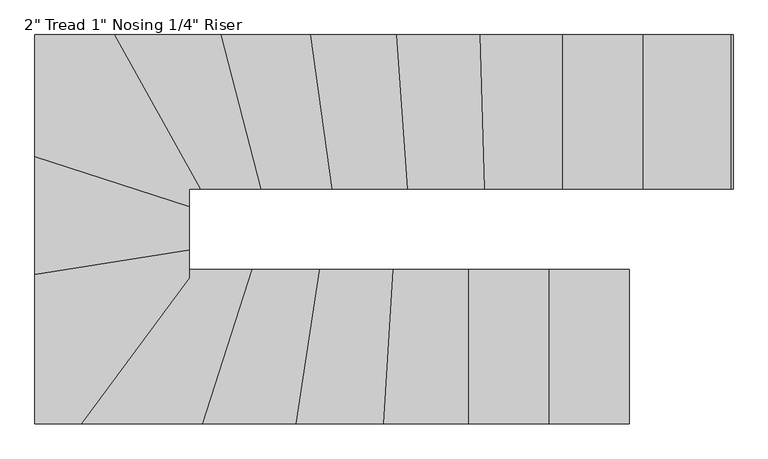
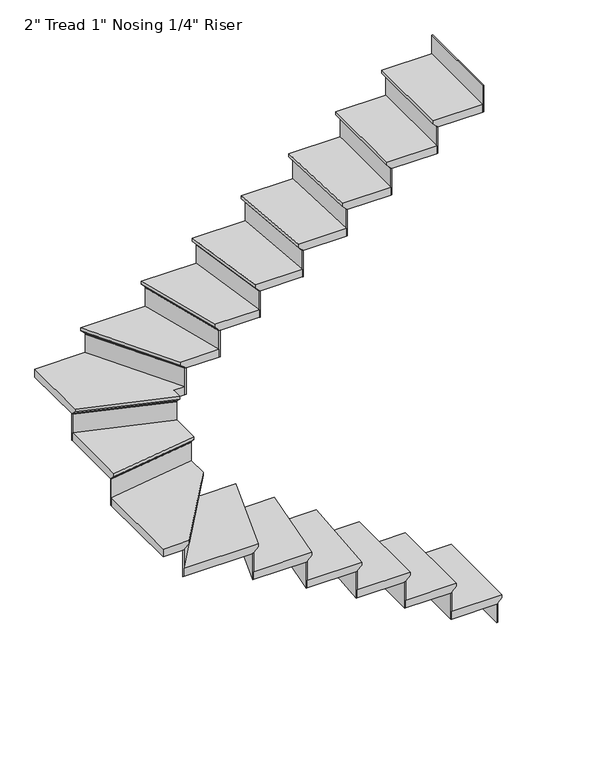
"""IFC4 building model written with IfcOpenShell, lengths in millimetres: stair flight geometry."""

from ifc_helpers import new_model, si_unit, origin, place, context, project, spatial, faceted_brep, source, transform, mapped, element, save


def stair_flight_033e9654(model_context):
    return source(origin(), model_context, "Body", "Brep", [
        faceted_brep([(-264.8831579, 264.4433073, 6551.0833333), (-264.8831579, 264.4433073, 6570.1333333), (-264.8831579, -271.8029286, 6570.1333333), (-264.8831579, -271.8029286, 6551.0833333), (-290.2831579, 264.4433073, 6525.6833333), (-290.2831579, -271.8029286, 6525.6833333), (-569.6831579, 264.4433073, 6570.1333333), (-569.6831579, -271.8029286, 6570.1333333), (-290.2831579, -271.8029286, 6519.3333333), (-569.6831579, -271.8029286, 6519.3333333), (-569.6831579, 264.4433073, 6519.3333333), (-290.2831579, 264.4433073, 6519.3333333)], [[[0, 1, 2, 3]], [[4, 0, 3, 5]], [[2, 1, 6, 7]], [[8, 9, 10, 11]], [[2, 7, 9, 8, 5, 3]], [[8, 11, 4, 5]], [[6, 1, 0, 4, 11, 10]], [[7, 6, 10, 9]]]),
        faceted_brep([(-290.2831579, 264.4433073, 6519.3333333), (-290.2831579, 264.4433073, 6400.8), (-296.6331579, 264.4433073, 6400.8), (-296.6331579, 264.4433073, 6519.3333333), (-290.2831579, -271.8029286, 6519.3333333), (-296.6331579, -271.8029286, 6519.3333333), (-296.6331579, -271.8029286, 6400.8), (-290.2831579, -271.8029286, 6400.8)], [[[0, 1, 2, 3]], [[4, 5, 6, 7]], [[1, 0, 4, 7]], [[2, 1, 7, 6]], [[3, 2, 6, 5]], [[0, 3, 5, 4]]]),
        faceted_brep([(-569.6831579, 264.4433073, 6688.6666667), (-569.6831579, 264.4433073, 6519.3333333), (-576.0331579, 264.4433073, 6519.3333333), (-576.0331579, 264.4433073, 6688.6666667), (-569.6831579, -271.8029286, 6688.6666667), (-576.0331579, -271.8029286, 6688.6666667), (-576.0331579, -271.8029286, 6519.3333333), (-569.6831579, -271.8029286, 6519.3333333)], [[[0, 1, 2, 3]], [[4, 5, 6, 7]], [[1, 0, 4, 7]], [[2, 1, 7, 6]], [[3, 2, 6, 5]], [[0, 3, 5, 4]]]),
        faceted_brep([(-544.2831579, -271.8029286, 6739.4666667), (-544.2831579, 264.4433073, 6739.4666667), (-849.0831579, 264.4433073, 6739.4666667), (-849.0831579, -271.8029286, 6739.4666667), (-569.6831579, -271.8029286, 6688.6666667), (-849.0831579, -271.8029286, 6688.6666667), (-849.0831579, 264.4433073, 6688.6666667), (-569.6831579, 264.4433073, 6688.6666667), (-569.6831579, -271.8029286, 6695.0166667), (-544.2831579, -271.8029286, 6720.4166667), (-569.6831579, 264.4433073, 6695.0166667), (-544.2831579, 264.4433073, 6720.4166667)], [[[0, 1, 2, 3]], [[4, 5, 6, 7]], [[0, 3, 5, 4, 8, 9]], [[4, 7, 10, 8]], [[2, 1, 11, 10, 7, 6]], [[3, 2, 6, 5]], [[11, 1, 0, 9]], [[10, 11, 9, 8]]]),
        faceted_brep([(-849.0831579, 264.4433073, 6858.0), (-849.0831579, 264.4433073, 6688.6666667), (-855.4331579, 264.4433073, 6688.6666667), (-855.4331579, 264.4433073, 6858.0), (-849.0831579, -271.8029286, 6858.0), (-855.4331579, -271.8029286, 6858.0), (-855.4331579, -271.8029286, 6688.6666667), (-849.0831579, -271.8029286, 6688.6666667)], [[[0, 1, 2, 3]], [[4, 5, 6, 7]], [[1, 0, 4, 7]], [[2, 1, 7, 6]], [[3, 2, 6, 5]], [[0, 3, 5, 4]]]),
        faceted_brep([(-823.6831579, -271.8029286, 6908.8), (-823.6831579, 264.4433073, 6908.8), (-1112.6009003, 264.4433073, 6908.8), (-1144.4549627, -271.8029286, 6908.8), (-849.0831579, -271.8029286, 6858.0), (-1144.4549627, -271.8029286, 6858.0), (-1112.6009003, 264.4433073, 6858.0), (-849.0831579, 264.4433073, 6858.0), (-849.0831579, -271.8029286, 6864.35), (-823.6831579, -271.8029286, 6889.75), (-849.0831579, 264.4433073, 6864.35), (-823.6831579, 264.4433073, 6889.75)], [[[0, 1, 2, 3]], [[4, 5, 6, 7]], [[0, 3, 5, 4, 8, 9]], [[4, 7, 10, 8]], [[2, 1, 11, 10, 7, 6]], [[3, 2, 6, 5]], [[11, 1, 0, 9]], [[10, 11, 9, 8]]]),
        faceted_brep([(-1112.6009003, 264.4433073, 7027.3333333), (-1112.6009003, 264.4433073, 6858.0), (-1118.9620938, 264.4433073, 6858.0), (-1118.9620938, 264.4433073, 7027.3333333), (-1144.4549627, -271.8029286, 7027.3333333), (-1150.8161561, -271.8029286, 7027.3333333), (-1150.8161561, -271.8029286, 6858.0), (-1144.4549627, -271.8029286, 6858.0)], [[[0, 1, 2, 3]], [[4, 5, 6, 7]], [[1, 0, 4, 7]], [[2, 1, 7, 6]], [[3, 2, 6, 5]], [[0, 3, 5, 4]]]),
        faceted_brep([(-1119.0101891, -271.8029286, 7078.1333333), (-1087.1561267, 264.4433073, 7078.1333333), (-1367.1376579, 264.4433073, 7078.1333333), (-1449.2203373, -271.8029286, 7078.1333333), (-1144.4549627, -271.8029286, 7027.3333333), (-1449.2203373, -271.8029286, 7027.3333333), (-1367.1376579, 264.4433073, 7027.3333333), (-1112.6009003, 264.4433073, 7027.3333333), (-1144.4549627, -271.8029286, 7033.6833333), (-1119.0101891, -271.8029286, 7059.0833333), (-1112.6009003, 264.4433073, 7033.6833333), (-1087.1561267, 264.4433073, 7059.0833333)], [[[0, 1, 2, 3]], [[4, 5, 6, 7]], [[0, 3, 5, 4, 8, 9]], [[4, 7, 10, 8]], [[2, 1, 11, 10, 7, 6]], [[3, 2, 6, 5]], [[11, 1, 0, 9]], [[10, 11, 9, 8]]]),
        faceted_brep([(-1367.1376579, 264.4433073, 7196.6666667), (-1367.1376579, 264.4433073, 7027.3333333), (-1373.5616178, 264.4433073, 7027.3333333), (-1373.5616178, 264.4433073, 7196.6666667), (-1449.2203373, -271.8029286, 7196.6666667), (-1455.6442972, -271.8029286, 7196.6666667), (-1455.6442972, -271.8029286, 7027.3333333), (-1449.2203373, -271.8029286, 7027.3333333)], [[[0, 1, 2, 3]], [[4, 5, 6, 7]], [[1, 0, 4, 7]], [[2, 1, 7, 6]], [[3, 2, 6, 5]], [[0, 3, 5, 4]]]),
        faceted_brep([(-1423.5244976, -271.8029286, 7247.4666667), (-1341.4418182, 264.4433073, 7247.4666667), (-1602.0584075, 264.4433073, 7247.4666667), (-1775.0869242, -271.8029286, 7247.4666667), (-1449.2203373, -271.8029286, 7196.6666667), (-1775.0869242, -271.8029286, 7196.6666667), (-1602.0584075, 264.4433073, 7196.6666667), (-1367.1376579, 264.4433073, 7196.6666667), (-1449.2203373, -271.8029286, 7203.0166667), (-1423.5244976, -271.8029286, 7228.4166667), (-1367.1376579, 264.4433073, 7203.0166667), (-1341.4418182, 264.4433073, 7228.4166667)], [[[0, 1, 2, 3]], [[4, 5, 6, 7]], [[0, 3, 5, 4, 8, 9]], [[4, 7, 10, 8]], [[2, 1, 11, 10, 7, 6]], [[3, 2, 6, 5]], [[11, 1, 0, 9]], [[10, 11, 9, 8]]]),
        faceted_brep([(-1602.0584075, 264.4433073, 7366.0), (-1602.0584075, 264.4433073, 7196.6666667), (-1608.7307845, 264.4433073, 7196.6666667), (-1608.7307845, 264.4433073, 7366.0), (-1775.0869242, -271.8029286, 7366.0), (-1781.7593012, -271.8029286, 7366.0), (-1781.7593012, -271.8029286, 7196.6666667), (-1775.0869242, -271.8029286, 7196.6666667)], [[[0, 1, 2, 3]], [[4, 5, 6, 7]], [[1, 0, 4, 7]], [[2, 1, 7, 6]], [[3, 2, 6, 5]], [[0, 3, 5, 4]]]),
        faceted_brep([(-1748.3974163, -271.8029286, 7416.8), (-1575.3688995, 264.4433073, 7416.8), (-1792.6148498, 264.4433073, 7416.8), (-1792.6148498, 277.721026, 7416.8), (-2200.2950016, -271.8029286, 7416.8), (-1775.0869242, -271.8029286, 7366.0), (-2200.2950016, -271.8029286, 7366.0), (-1792.6148498, 277.721026, 7366.0), (-1792.6148498, 264.4433073, 7366.0), (-1602.0584075, 264.4433073, 7366.0), (-1775.0869242, -271.8029286, 7372.35), (-1748.3974163, -271.8029286, 7397.75), (-1602.0584075, 264.4433073, 7372.35), (-1575.3688995, 264.4433073, 7397.75)], [[[0, 1, 2, 3, 4]], [[5, 6, 7, 8, 9]], [[0, 4, 6, 5, 10, 11]], [[5, 9, 12, 10]], [[2, 1, 13, 12, 9, 8]], [[4, 3, 7, 6]], [[13, 1, 0, 11]], [[12, 13, 11, 10]], [[3, 2, 8, 7]]]),
        faceted_brep([(-1792.6148498, 277.721026, 7535.3333333), (-1792.6148498, 277.721026, 7366.0), (-1792.6148498, 288.3786511, 7366.0), (-1792.6148498, 288.3786511, 7535.3333333), (-2200.2950016, -271.8029286, 7535.3333333), (-2208.2016673, -271.8029286, 7535.3333333), (-2208.2016673, -271.8029286, 7366.0), (-2200.2950016, -271.8029286, 7366.0)], [[[0, 1, 2, 3]], [[4, 5, 6, 7]], [[1, 0, 4, 7]], [[2, 1, 7, 6]], [[3, 2, 6, 5]], [[0, 3, 5, 4]]]),
        faceted_brep([(-2328.8610857, 272.9225747, 7586.1333333), (-2328.8610857, -271.8029286, 7586.1333333), (-2168.6683387, -271.8029286, 7586.1333333), (-1792.6148498, 235.0905257, 7586.1333333), (-1792.6148498, 358.7948785, 7586.1333333), (-2328.8610857, -271.8029286, 7535.3333333), (-2328.8610857, 272.9225747, 7535.3333333), (-1792.6148498, 358.7948785, 7535.3333333), (-1792.6148498, 277.721026, 7535.3333333), (-2200.2950016, -271.8029286, 7535.3333333), (-2200.2950016, -271.8029286, 7541.6833333), (-2168.6683387, -271.8029286, 7567.0833333), (-1792.6148498, 277.721026, 7541.6833333), (-1792.6148498, 235.0905257, 7567.0833333)], [[[0, 1, 2, 3, 4]], [[5, 6, 7, 8, 9]], [[1, 0, 6, 5]], [[2, 1, 5, 9, 10, 11]], [[9, 8, 12, 10]], [[4, 3, 13, 12, 8, 7]], [[0, 4, 7, 6]], [[13, 3, 2, 11]], [[12, 13, 11, 10]]]),
        faceted_brep([(-1792.6148498, 358.7948785, 7704.6666667), (-1792.6148498, 358.7948785, 7535.3333333), (-1792.6148498, 365.2257813, 7535.3333333), (-1792.6148498, 365.2257813, 7704.6666667), (-2328.8610857, 272.9225747, 7704.6666667), (-2328.8610857, 279.3534775, 7704.6666667), (-2328.8610857, 279.3534775, 7535.3333333), (-2328.8610857, 272.9225747, 7535.3333333)], [[[0, 1, 2, 3]], [[4, 5, 6, 7]], [[1, 0, 4, 7]], [[2, 1, 7, 6]], [[3, 2, 6, 5]], [[0, 3, 5, 4]]]),
        faceted_brep([(-2328.8610857, 247.1989634, 7755.4666667), (-1792.6148498, 333.0712672, 7755.4666667), (-1792.6148498, 510.0383883, 7755.4666667), (-2328.8610857, 683.2061106, 7755.4666667), (-2328.8610857, 272.9225747, 7704.6666667), (-2328.8610857, 683.2061106, 7704.6666667), (-1792.6148498, 510.0383883, 7704.6666667), (-1792.6148498, 358.7948785, 7704.6666667), (-2328.8610857, 272.9225747, 7711.0166667), (-2328.8610857, 247.1989634, 7736.4166667), (-1792.6148498, 358.7948785, 7711.0166667), (-1792.6148498, 333.0712672, 7736.4166667)], [[[0, 1, 2, 3]], [[4, 5, 6, 7]], [[0, 3, 5, 4, 8, 9]], [[4, 7, 10, 8]], [[3, 2, 6, 5]], [[11, 1, 0, 9]], [[10, 11, 9, 8]], [[2, 1, 11, 10, 7, 6]]]),
        faceted_brep([(-1792.6148498, 510.0383883, 7874.0), (-1792.6148498, 510.0383883, 7704.6666667), (-1792.6148498, 516.7112716, 7704.6666667), (-1792.6148498, 516.7112716, 7874.0), (-2328.8610857, 683.2061106, 7874.0), (-2328.8610857, 689.878994, 7874.0), (-2328.8610857, 689.878994, 7704.6666667), (-2328.8610857, 683.2061106, 7704.6666667)], [[[0, 1, 2, 3]], [[4, 5, 6, 7]], [[1, 0, 4, 7]], [[2, 1, 7, 6]], [[3, 2, 6, 5]], [[0, 3, 5, 4]]]),
        faceted_brep([(-2021.9568272, 1080.0895433, 7924.8), (-2328.8610857, 1080.0895433, 7924.8), (-2328.8610857, 656.5145772, 7924.8), (-1792.6148498, 483.3468548, 7924.8), (-1792.6148498, 543.8433073, 7924.8), (-1724.5287393, 543.8433073, 7924.8), (-2328.8610857, 1080.0895433, 7874.0), (-2021.9568272, 1080.0895433, 7874.0), (-1724.5287393, 543.8433073, 7874.0), (-1792.6148498, 543.8433073, 7874.0), (-1792.6148498, 510.0383883, 7874.0), (-2328.8610857, 683.2061106, 7874.0), (-1792.6148498, 510.0383883, 7880.35), (-2328.8610857, 683.2061106, 7880.35), (-1792.6148498, 483.3468548, 7905.75), (-2328.8610857, 656.5145772, 7905.75)], [[[0, 1, 2, 3, 4, 5]], [[6, 7, 8, 9, 10, 11]], [[1, 0, 7, 6]], [[11, 10, 12, 13]], [[4, 3, 14, 12, 10, 9]], [[0, 5, 8, 7]], [[14, 3, 2, 15]], [[12, 14, 15, 13]], [[2, 1, 6, 11, 13, 15]], [[5, 4, 9, 8]]]),
        faceted_brep([(-1724.5287393, 543.8433073, 8043.3333333), (-1724.5287393, 543.8433073, 7874.0), (-1717.2673962, 543.8433073, 7874.0), (-1717.2673962, 543.8433073, 8043.3333333), (-2021.9568272, 1080.0895433, 8043.3333333), (-2014.6954841, 1080.0895433, 8043.3333333), (-2014.6954841, 1080.0895433, 7874.0), (-2021.9568272, 1080.0895433, 7874.0)], [[[0, 1, 2, 3]], [[4, 5, 6, 7]], [[1, 0, 4, 7]], [[2, 1, 7, 6]], [[3, 2, 6, 5]], [[0, 3, 5, 4]]]),
        faceted_brep([(-2051.0021996, 1080.0895433, 8094.1333333), (-1753.5741117, 543.8433073, 8094.1333333), (-1517.487325, 543.8433073, 8094.1333333), (-1656.0375972, 1080.0895433, 8094.1333333), (-2021.9568272, 1080.0895433, 8043.3333333), (-1656.0375972, 1080.0895433, 8043.3333333), (-1517.487325, 543.8433073, 8043.3333333), (-1724.5287393, 543.8433073, 8043.3333333), (-2021.9568272, 1080.0895433, 8049.6833333), (-2051.0021996, 1080.0895433, 8075.0833333), (-1724.5287393, 543.8433073, 8049.6833333), (-1753.5741117, 543.8433073, 8075.0833333)], [[[0, 1, 2, 3]], [[4, 5, 6, 7]], [[0, 3, 5, 4, 8, 9]], [[4, 7, 10, 8]], [[2, 1, 11, 10, 7, 6]], [[3, 2, 6, 5]], [[11, 1, 0, 9]], [[10, 11, 9, 8]]]),
        faceted_brep([(-1517.487325, 543.8433073, 8212.6666667), (-1517.487325, 543.8433073, 8043.3333333), (-1510.9288005, 543.8433073, 8043.3333333), (-1510.9288005, 543.8433073, 8212.6666667), (-1656.0375972, 1080.0895433, 8212.6666667), (-1649.4790727, 1080.0895433, 8212.6666667), (-1649.4790727, 1080.0895433, 8043.3333333), (-1656.0375972, 1080.0895433, 8043.3333333)], [[[0, 1, 2, 3]], [[4, 5, 6, 7]], [[1, 0, 4, 7]], [[2, 1, 7, 6]], [[3, 2, 6, 5]], [[0, 3, 5, 4]]]),
        faceted_brep([(-1682.2716952, 1080.0895433, 8263.4666667), (-1543.721423, 543.8433073, 8263.4666667), (-1271.2041837, 543.8433073, 8263.4666667), (-1344.713853, 1080.0895433, 8263.4666667), (-1656.0375972, 1080.0895433, 8212.6666667), (-1344.713853, 1080.0895433, 8212.6666667), (-1271.2041837, 543.8433073, 8212.6666667), (-1517.487325, 543.8433073, 8212.6666667), (-1656.0375972, 1080.0895433, 8219.0166667), (-1682.2716952, 1080.0895433, 8244.4166667), (-1517.487325, 543.8433073, 8219.0166667), (-1543.721423, 543.8433073, 8244.4166667)], [[[0, 1, 2, 3]], [[4, 5, 6, 7]], [[0, 3, 5, 4, 8, 9]], [[4, 7, 10, 8]], [[2, 1, 11, 10, 7, 6]], [[3, 2, 6, 5]], [[11, 1, 0, 9]], [[10, 11, 9, 8]]]),
        faceted_brep([(-1271.2041837, 543.8433073, 8382.0), (-1271.2041837, 543.8433073, 8212.6666667), (-1264.7947985, 543.8433073, 8212.6666667), (-1264.7947985, 543.8433073, 8382.0), (-1344.713853, 1080.0895433, 8382.0), (-1338.3044678, 1080.0895433, 8382.0), (-1338.3044678, 1080.0895433, 8212.6666667), (-1344.713853, 1080.0895433, 8212.6666667)], [[[0, 1, 2, 3]], [[4, 5, 6, 7]], [[1, 0, 4, 7]], [[2, 1, 7, 6]], [[3, 2, 6, 5]], [[0, 3, 5, 4]]]),
        faceted_brep([(-1370.3513937, 1080.0895433, 8432.8), (-1296.8417245, 543.8433073, 8432.8), (-1009.7763573, 543.8433073, 8432.8), (-1047.6899509, 1080.0895433, 8432.8), (-1344.713853, 1080.0895433, 8382.0), (-1047.6899509, 1080.0895433, 8382.0), (-1009.7763573, 543.8433073, 8382.0), (-1271.2041837, 543.8433073, 8382.0), (-1344.713853, 1080.0895433, 8388.35), (-1370.3513937, 1080.0895433, 8413.75), (-1271.2041837, 543.8433073, 8388.35), (-1296.8417245, 543.8433073, 8413.75)], [[[0, 1, 2, 3]], [[4, 5, 6, 7]], [[0, 3, 5, 4, 8, 9]], [[4, 7, 10, 8]], [[2, 1, 11, 10, 7, 6]], [[3, 2, 6, 5]], [[11, 1, 0, 9]], [[10, 11, 9, 8]]]),
        faceted_brep([(-1009.7763573, 543.8433073, 8551.3333333), (-1009.7763573, 543.8433073, 8382.0), (-1003.4105061, 543.8433073, 8382.0), (-1003.4105061, 543.8433073, 8551.3333333), (-1047.6899509, 1080.0895433, 8551.3333333), (-1041.3240997, 1080.0895433, 8551.3333333), (-1041.3240997, 1080.0895433, 8382.0), (-1047.6899509, 1080.0895433, 8382.0)], [[[0, 1, 2, 3]], [[4, 5, 6, 7]], [[1, 0, 4, 7]], [[2, 1, 7, 6]], [[3, 2, 6, 5]], [[0, 3, 5, 4]]]),
        faceted_brep([(-1073.1533559, 1080.0895433, 8602.1333333), (-1035.2397623, 543.8433073, 8602.1333333), (-741.6570892, 543.8433073, 8602.1333333), (-757.1149275, 1080.0895433, 8602.1333333), (-1047.6899509, 1080.0895433, 8551.3333333), (-757.1149275, 1080.0895433, 8551.3333333), (-741.6570892, 543.8433073, 8551.3333333), (-1009.7763573, 543.8433073, 8551.3333333), (-1047.6899509, 1080.0895433, 8557.6833333), (-1073.1533559, 1080.0895433, 8583.0833333), (-1009.7763573, 543.8433073, 8557.6833333), (-1035.2397623, 543.8433073, 8583.0833333)], [[[0, 1, 2, 3]], [[4, 5, 6, 7]], [[0, 3, 5, 4, 8, 9]], [[4, 7, 10, 8]], [[2, 1, 11, 10, 7, 6]], [[3, 2, 6, 5]], [[11, 1, 0, 9]], [[10, 11, 9, 8]]]),
        faceted_brep([(-741.6570892, 543.8433073, 8720.6666667), (-741.6570892, 543.8433073, 8551.3333333), (-735.3044516, 543.8433073, 8551.3333333), (-735.3044516, 543.8433073, 8720.6666667), (-757.1149275, 1080.0895433, 8720.6666667), (-750.7622898, 1080.0895433, 8720.6666667), (-750.7622898, 1080.0895433, 8551.3333333), (-757.1149275, 1080.0895433, 8551.3333333)], [[[0, 1, 2, 3]], [[4, 5, 6, 7]], [[1, 0, 4, 7]], [[2, 1, 7, 6]], [[3, 2, 6, 5]], [[0, 3, 5, 4]]]),
        faceted_brep([(-782.5254783, 1080.0895433, 8771.4666667), (-767.06764, 543.8433073, 8771.4666667), (-469.9965591, 543.8433073, 8771.4666667), (-469.9965591, 1080.0895433, 8771.4666667), (-757.1149275, 1080.0895433, 8720.6666667), (-469.9965591, 1080.0895433, 8720.6666667), (-469.9965591, 543.8433073, 8720.6666667), (-741.6570892, 543.8433073, 8720.6666667), (-757.1149275, 1080.0895433, 8727.0166667), (-782.5254783, 1080.0895433, 8752.4166667), (-741.6570892, 543.8433073, 8727.0166667), (-767.06764, 543.8433073, 8752.4166667)], [[[0, 1, 2, 3]], [[4, 5, 6, 7]], [[0, 3, 5, 4, 8, 9]], [[4, 7, 10, 8]], [[2, 1, 11, 10, 7, 6]], [[3, 2, 6, 5]], [[11, 1, 0, 9]], [[10, 11, 9, 8]]]),
        faceted_brep([(-469.9965591, 543.8433073, 8890.0), (-469.9965591, 543.8433073, 8720.6666667), (-463.6465591, 543.8433073, 8720.6666667), (-463.6465591, 543.8433073, 8890.0), (-469.9965591, 1080.0895433, 8890.0), (-463.6465591, 1080.0895433, 8890.0), (-463.6465591, 1080.0895433, 8720.6666667), (-469.9965591, 1080.0895433, 8720.6666667)], [[[0, 1, 2, 3]], [[4, 5, 6, 7]], [[1, 0, 4, 7]], [[2, 1, 7, 6]], [[3, 2, 6, 5]], [[0, 3, 5, 4]]]),
        faceted_brep([(-495.3965591, 1080.0895433, 8940.8), (-495.3965591, 543.8433073, 8940.8), (-190.5965591, 543.8433073, 8940.8), (-190.5965591, 1080.0895433, 8940.8), (-469.9965591, 1080.0895433, 8890.0), (-190.5965591, 1080.0895433, 8890.0), (-190.5965591, 543.8433073, 8890.0), (-469.9965591, 543.8433073, 8890.0), (-469.9965591, 1080.0895433, 8896.35), (-495.3965591, 1080.0895433, 8921.75), (-469.9965591, 543.8433073, 8896.35), (-495.3965591, 543.8433073, 8921.75)], [[[0, 1, 2, 3]], [[4, 5, 6, 7]], [[0, 3, 5, 4, 8, 9]], [[4, 7, 10, 8]], [[2, 1, 11, 10, 7, 6]], [[3, 2, 6, 5]], [[11, 1, 0, 9]], [[10, 11, 9, 8]]]),
        faceted_brep([(-190.5965591, 543.8433073, 9059.3333333), (-190.5965591, 543.8433073, 8890.0), (-184.2465591, 543.8433073, 8890.0), (-184.2465591, 543.8433073, 9059.3333333), (-190.5965591, 1080.0895433, 9059.3333333), (-184.2465591, 1080.0895433, 9059.3333333), (-184.2465591, 1080.0895433, 8890.0), (-190.5965591, 1080.0895433, 8890.0)], [[[0, 1, 2, 3]], [[4, 5, 6, 7]], [[1, 0, 4, 7]], [[2, 1, 7, 6]], [[3, 2, 6, 5]], [[0, 3, 5, 4]]]),
        faceted_brep([(88.8034409, 543.8433073, 9228.6666667), (88.8034409, 543.8433073, 9059.3333333), (95.1534409, 543.8433073, 9059.3333333), (95.1534409, 543.8433073, 9228.6666667), (88.8034409, 1080.0895433, 9228.6666667), (95.1534409, 1080.0895433, 9228.6666667), (95.1534409, 1080.0895433, 9059.3333333), (88.8034409, 1080.0895433, 9059.3333333)], [[[0, 1, 2, 3]], [[4, 5, 6, 7]], [[1, 0, 4, 7]], [[2, 1, 7, 6]], [[3, 2, 6, 5]], [[0, 3, 5, 4]]]),
        faceted_brep([(-215.9965591, 1080.0895433, 9110.1333333), (-215.9965591, 543.8433073, 9110.1333333), (88.8034409, 543.8433073, 9110.1333333), (88.8034409, 1080.0895433, 9110.1333333), (-190.5965591, 1080.0895433, 9059.3333333), (88.8034409, 1080.0895433, 9059.3333333), (88.8034409, 543.8433073, 9059.3333333), (-190.5965591, 543.8433073, 9059.3333333), (-190.5965591, 1080.0895433, 9065.6833333), (-215.9965591, 1080.0895433, 9091.0833333), (-190.5965591, 543.8433073, 9065.6833333), (-215.9965591, 543.8433073, 9091.0833333)], [[[0, 1, 2, 3]], [[4, 5, 6, 7]], [[0, 3, 5, 4, 8, 9]], [[4, 7, 10, 8]], [[2, 1, 11, 10, 7, 6]], [[3, 2, 6, 5]], [[11, 1, 0, 9]], [[10, 11, 9, 8]]]),
    ])


if __name__ == "__main__":
    model = new_model("IFC4")
    model_context = context("Model", 3, world=origin())
    ifc_project = project(units=[si_unit("LENGTHUNIT", "METRE", prefix="MILLI")], contexts=[model_context])
    site = spatial("IfcSite", under=ifc_project)
    building = spatial("IfcBuilding", under=site)
    placement = place(None, origin())
    stair_flight_shape = stair_flight_033e9654(model_context)
    element("IfcStairFlight", 1, ObjectType="2\" Tread 1\" Nosing 1/4\" Riser", at=placement, inside=building, context=model_context, shape_type="MappedRepresentation", body=[
        mapped(stair_flight_shape, transform((0.0, 0.0, 0.0), x_axis=(1.0, 0.0, 0.0), y_axis=(0.0, 1.0, 0.0), z_axis=(0.0, 0.0, 1.0))),
    ])
    save(model, "model.ifc")
